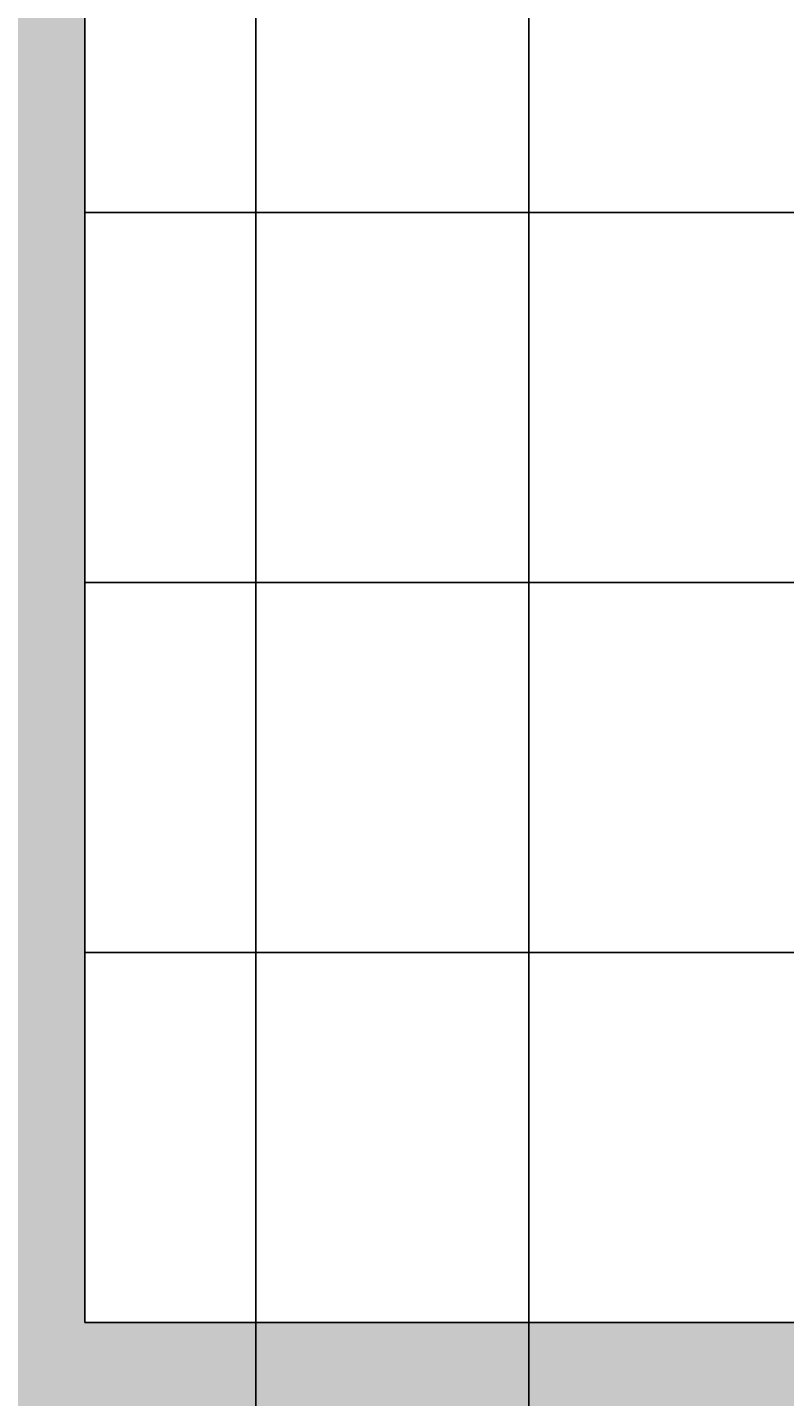
# Model space of a CAD drawing. Units: inches. Extents: x 2231 to 2461, y 2045 to 2455.
# Tile 58 of 95: x 2395 to 2416, y 2185 to 2222. Entities that reach past the tile are written whole.
import ezdxf

# ---------------------------------------------------------------- set-up
doc = ezdxf.new("R2010")
doc.units = ezdxf.units.IN
doc.layers.add('A-ANNO-DIMS', color=2, linetype='Continuous', lineweight=18)
doc.layers.add('A-FLOR-STRS', color=7, linetype='Continuous', lineweight=25)
doc.layers.add('A-WALL-PATT', color=18, linetype='Continuous', lineweight=13, true_color=0x000000)
doc.styles.get("Standard").update_dxf_attribs({"font": 'arial.ttf'})
doc.dimstyles.get("Standard").update_dxf_attribs({"dimtxt": 0.18, "dimasz": 0.18, "dimexe": 0.18, "dimexo": 0.0625, "dimgap": 0.09, "dimtad": 0, "dimtih": 1, "dimtoh": 1, "dimdec": 4, "dimzin": 0, "dimdsep": 46, "dimtxsty": 'Standard', "dimcen": 0.09, "dimadec": 0, "dimazin": 0, "dimtfac": 1, "dimtdec": 4, "dimtofl": 0, "dimtmove": 0, "dimatfit": 3, "dimfxl": 1, "dimtolj": 1, "dimtzin": 0, "dimarcsym": 0})

# ---------------------------------------------------------------- blocks, each defined once
blk = doc.blocks.new('*D59')
at = {"layer": 'A-ANNO-DIMS', "color": 0, "lineweight": -2, "transparency": 16777216}
for p, q in [((2408.794, 2182.895), (2408.794, 2454.645)), ((2432.794, 2182.895), (2432.794, 2454.645)), ((2408.974, 2454.465), (2420.573, 2454.465)), ((2432.614, 2454.465), (2421.014, 2454.465))]:
    blk.add_line(p, q, dxfattribs=at)
at = {"layer": 'A-ANNO-DIMS', "color": 0, "transparency": 16777216}
for points in [[(2408.974, 2454.495), (2408.974, 2454.435), (2408.794, 2454.465)], [(2432.614, 2454.495), (2432.614, 2454.435), (2432.794, 2454.465)]]:
    blk.add_solid(points, dxfattribs=at)
at = {"layer": 'Defpoints', "color": 0, "transparency": 16777216}
for p in [(2432.794, 2454.465), (2408.794, 2182.833), (2432.794, 2182.833)]:
    blk.add_point(p, dxfattribs=at)
at = {"layer": 'A-ANNO-DIMS', "color": 0, "transparency": 16777216, "insert": (2420.794, 2454.465), "char_height": 0.18, "attachment_point": 5}
blk.add_mtext('\\A1;24', dxfattribs=at)
blk = doc.blocks.new('*D66')
at = {"layer": 'A-ANNO-DIMS', "color": 0, "lineweight": -2, "transparency": 16777216}
for p, q in [((2348.189, 2096.895), (2348.189, 2454.645)), ((2408.794, 2096.895), (2408.794, 2454.645)), ((2348.369, 2454.465), (2378.167, 2454.465)), ((2408.614, 2454.465), (2378.815, 2454.465))]:
    blk.add_line(p, q, dxfattribs=at)
at = {"layer": 'A-ANNO-DIMS', "color": 0, "transparency": 16777216}
for points in [[(2348.369, 2454.495), (2348.369, 2454.435), (2348.189, 2454.465)], [(2408.614, 2454.495), (2408.614, 2454.435), (2408.794, 2454.465)]]:
    blk.add_solid(points, dxfattribs=at)
at = {"layer": 'Defpoints', "color": 0, "transparency": 16777216}
for p in [(2408.794, 2454.465), (2348.189, 2096.833), (2408.794, 2096.833)]:
    blk.add_point(p, dxfattribs=at)
at = {"layer": 'A-ANNO-DIMS', "color": 0, "transparency": 16777216, "insert": (2378.491, 2454.465), "char_height": 0.18, "attachment_point": 5}
blk.add_mtext('\\A1;60.6', dxfattribs=at)
blk = doc.blocks.new('*D71')
at = {"layer": 'A-ANNO-DIMS', "color": 0, "lineweight": -2, "transparency": 16777216}
for p, q in [((2401.422, 2092.979), (2401.422, 2454.645)), ((2408.794, 2096.895), (2408.794, 2454.645)), ((2401.602, 2454.465), (2404.732, 2454.465)), ((2408.614, 2454.465), (2405.483, 2454.465))]:
    blk.add_line(p, q, dxfattribs=at)
at = {"layer": 'A-ANNO-DIMS', "color": 0, "transparency": 16777216}
for points in [[(2401.602, 2454.495), (2401.602, 2454.435), (2401.422, 2454.465)], [(2408.614, 2454.495), (2408.614, 2454.435), (2408.794, 2454.465)]]:
    blk.add_solid(points, dxfattribs=at)
at = {"layer": 'Defpoints', "color": 0, "transparency": 16777216}
for p in [(2408.794, 2454.465), (2408.794, 2096.833), (2401.422, 2092.917)]:
    blk.add_point(p, dxfattribs=at)
at = {"layer": 'A-ANNO-DIMS', "color": 0, "transparency": 16777216, "insert": (2405.108, 2454.465), "char_height": 0.18, "attachment_point": 5}
blk.add_mtext('\\A1;7.371', dxfattribs=at)
blk = doc.blocks.new('*D72')
at = {"layer": 'A-ANNO-DIMS', "color": 0, "lineweight": -2, "transparency": 16777216}
for p, q in [((2384.543, 2145.12), (2384.543, 2454.645)), ((2408.794, 2150.677), (2408.794, 2454.645)), ((2384.723, 2454.465), (2396.272, 2454.465)), ((2408.614, 2454.465), (2397.064, 2454.465))]:
    blk.add_line(p, q, dxfattribs=at)
at = {"layer": 'A-ANNO-DIMS', "color": 0, "transparency": 16777216}
for points in [[(2384.723, 2454.495), (2384.723, 2454.435), (2384.543, 2454.465)], [(2408.614, 2454.495), (2408.614, 2454.435), (2408.794, 2454.465)]]:
    blk.add_solid(points, dxfattribs=at)
at = {"layer": 'Defpoints', "color": 0, "transparency": 16777216}
for p in [(2408.794, 2454.465), (2408.794, 2150.615), (2384.543, 2145.058)]:
    blk.add_point(p, dxfattribs=at)
at = {"layer": 'A-ANNO-DIMS', "color": 0, "transparency": 16777216, "insert": (2396.668, 2454.465), "char_height": 0.18, "attachment_point": 5}
blk.add_mtext('\\A1;24.25', dxfattribs=at)

msp = doc.modelspace()

# ---------------------------------------------------------------- hatches: boundary and pattern name
at = {"layer": 'A-WALL-PATT'}
h = msp.add_hatch(color=256, dxfattribs=at)
h.dxf.hatch_style = 1
h.paths.add_polyline_path([(2441.7935, 2269.1535), (2432.7935, 2269.1535), (2432.7935, 2186.8328), (2396.7935, 2186.8328), (2396.7935, 2286.8328), (2394.7935, 2286.8328), (2394.7935, 2186.8328), (2334.7935, 2186.8328), (2334.7935, 2182.8328), (2432.7935, 2182.8328), (2432.7935, 2072.8328), (2416.6639, 2072.8328), (2416.6639, 2063.8328), (2441.7935, 2063.8328)])
h.paths.add_polyline_path([(2368.6639, 2072.8328), (2367.04, 2072.8328), (2330.7942, 2072.8328), (2330.7397, 2063.8328), (2368.6639, 2063.8328)])
h.paths.add_polyline_path([(2300.7392, 2068.3328), (2300.7392, 2072.8328), (2298.7935, 2072.8328), (2294.7935, 2072.8328), (2258.7935, 2072.8328), (2258.7935, 2120.8328), (2294.7935, 2120.8328), (2298.7935, 2120.8328), (2298.7935, 2128.8328), (2294.7935, 2128.8328), (2294.7935, 2124.8328), (2258.7935, 2124.8328), (2258.7935, 2182.8328), (2294.7935, 2182.8328), (2294.7935, 2174.8328), (2298.7935, 2174.8328), (2298.7935, 2182.8328), (2304.7935, 2182.8328), (2304.7935, 2186.8328), (2258.7935, 2186.8328), (2258.7935, 2221.999), (2249.7935, 2221.999), (2249.7935, 2063.8328), (2300.7392, 2063.8328)])
h.paths.add_polyline_path([(2391.9338, 2435.8328), (2333.82, 2435.8328), (2333.82, 2426.8328), (2368.7935, 2426.8328), (2368.7935, 2374.9508), (2368.7935, 2370.8328), (2372.3935, 2370.8328), (2372.7935, 2370.8328), (2372.7935, 2426.8328), (2391.9338, 2426.8328)])
h.paths.add_polyline_path([(2441.7935, 2435.8328), (2415.9338, 2435.8328), (2415.9338, 2426.8328), (2432.7935, 2426.8328), (2432.7935, 2334.8328), (2372.7935, 2334.8328), (2372.7935, 2346.8328), (2368.7935, 2346.8328), (2368.7935, 2306.8328), (2360.7935, 2306.8328), (2360.7935, 2302.8328), (2368.7935, 2302.8328), (2372.7935, 2302.8328), (2372.7935, 2330.8328), (2432.7935, 2330.8328), (2432.7935, 2317.1535), (2441.7935, 2317.1535)])
h.paths.add_polyline_path([(2285.82, 2435.8328), (2249.7935, 2435.8328), (2249.7935, 2269.999), (2258.7935, 2269.999), (2258.7935, 2302.8328), (2318.8168, 2302.8328), (2330.7935, 2302.8328), (2330.7935, 2306.8328), (2258.7935, 2306.8328), (2258.7935, 2426.8328), (2285.82, 2426.8328)])

# ---------------------------------------------------------------- linework, layer by layer
at = {"layer": 'A-FLOR-STRS'}
for p, q in [((2396.7935, 2286.8328), (2396.7935, 2186.8328)), ((2396.7935, 2216.8328), (2432.7935, 2216.8328)), ((2396.7935, 2206.8328), (2432.7935, 2206.8328)), ((2396.7935, 2196.8328), (2432.7935, 2196.8328)), ((2396.7935, 2186.8328), (2432.7935, 2186.8328))]:
    msp.add_line(p, q, dxfattribs=at)

# ---------------------------------------------------------------- dimensions: what is measured, and where the dimension line sits
at = {"layer": 'A-ANNO-DIMS'}
for base, p1, p2, override, picture, middle in [((2408.7935, 2454.4653), (2348.1888, 2096.8328), (2408.7935, 2096.8328), {"dimdec": 1, "dimlfac": 1, "dimrnd": 0, "dimzin": 0, "dimdsep": 46, "dimlunit": 2}, '*D66', (2378.4912, 2454.4653)), ((2408.7935, 2454.4653), (2384.5428, 2145.0576), (2408.7935, 2150.6145), {"dimdec": 2, "dimlfac": 1, "dimrnd": 0, "dimzin": 0, "dimdsep": 46, "dimlunit": 2}, '*D72', (2396.6682, 2454.4653)), ((2408.7935, 2454.4653), (2401.4221, 2092.9167), (2408.7935, 2096.8328), {"dimdec": 3, "dimlfac": 1, "dimrnd": 0, "dimzin": 0, "dimdsep": 46, "dimlunit": 2}, '*D71', (2405.1078, 2454.4653)), ((2432.7935, 2454.4653), (2408.7935, 2182.8328), (2432.7935, 2182.8328), {"dimdec": 0, "dimlfac": 1, "dimrnd": 0, "dimzin": 0, "dimdsep": 46, "dimlunit": 2}, '*D59', (2420.7935, 2454.4653))]:
    dim = msp.add_linear_dim(base=base, p1=p1, p2=p2, dimstyle='Standard', override=override, dxfattribs=at)
    dim.commit()
    dim.dimension.update_dxf_attribs({"geometry": picture, "text_midpoint": middle})

doc.saveas('drawing.dxf')
